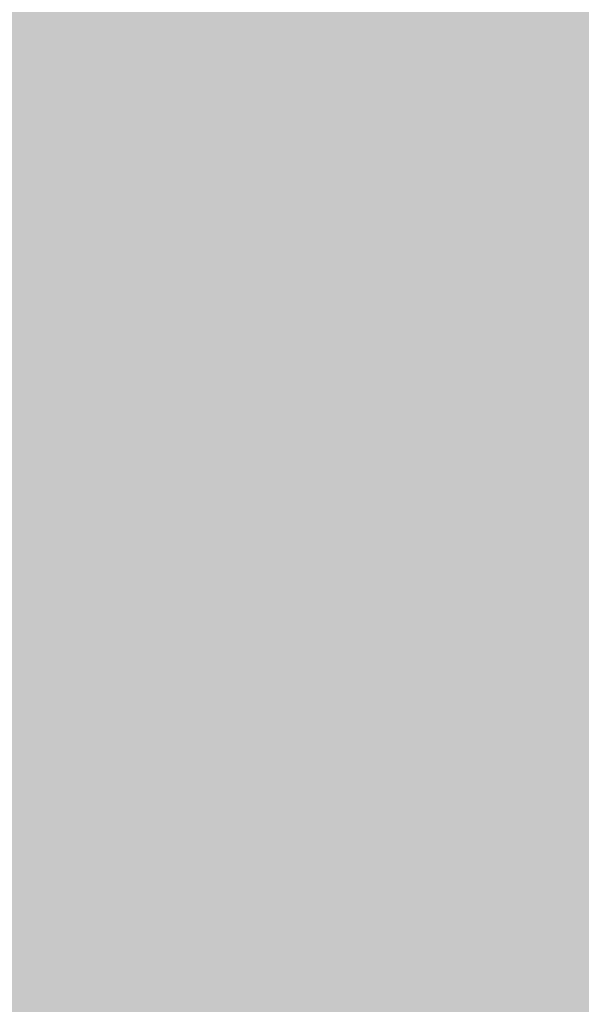
# Model space of a CAD drawing. Units: inches. Extents: x 2083 to 3317, y 1141 to 2115.
# Tile 186 of 256: x 3126.6699 to 3126.8176, y 1263.3548 to 1263.6134. Entities that reach past the tile are written whole.
import ezdxf

# ---------------------------------------------------------------- set-up
doc = ezdxf.new("R2010")
doc.units = ezdxf.units.IN
doc.layers.add('A-ANNO-DIMS', color=2, linetype='Continuous', lineweight=18)
doc.layers.add('A-WALL-PATT', color=251, linetype='Continuous', lineweight=13, true_color=0x636466)
doc.styles.get("Standard").update_dxf_attribs({"font": 'arial.ttf'})
doc.dimstyles.new('ISO-25', dxfattribs={"dimtxt": 12, "dimasz": 12, "dimexe": 1.25, "dimexo": 0.625, "dimtad": 1, "dimlunit": 3, "dimtxsty": 'Standard', "dimcen": 2.5, "dimadec": 0, "dimazin": 0, "dimtfac": 1, "dimtmove": 0, "dimatfit": 3, "dimfxl": 1, "dimarcsym": 0})

# ---------------------------------------------------------------- blocks, each defined once
blk = doc.blocks.new('*D26')
at = {"layer": 'A-ANNO-DIMS', "color": 0, "lineweight": -2, "transparency": 16777216}
for p, q in [((3088.98584, 1274.91509), (3088.98584, 1270.95196)), ((3111.24004, 1274.91509), (3111.24004, 1270.95196)), ((3076.98584, 1272.20196), (2840.26245, 1272.20196)), ((3111.24004, 1272.20196), (3088.98584, 1272.20196)), ((3123.24004, 1272.20196), (3135.24004, 1272.20196))]:
    blk.add_line(p, q, dxfattribs=at)
at = {"layer": 'A-ANNO-DIMS', "color": 0, "transparency": 16777216}
for points in [[(3076.98584, 1274.20196), (3076.98584, 1270.20196), (3088.98584, 1272.20196)], [(3123.24004, 1274.20196), (3123.24004, 1270.20196), (3111.24004, 1272.20196)]]:
    blk.add_solid(points, dxfattribs=at)
at = {"layer": 'Defpoints', "color": 0, "transparency": 16777216}
for p in [(3088.98584, 1275.54009), (3111.24004, 1275.54009), (3088.98584, 1272.20196)]:
    blk.add_point(p, dxfattribs=at)
at = {"layer": 'A-ANNO-DIMS', "color": 0, "transparency": 16777216, "insert": (2952.62415, 1279.0316), "char_height": 12, "attachment_point": 5}
blk.add_mtext('NIGHTSTAND 1\'-10 1/2" TYP.', dxfattribs=at)
blk = doc.blocks.new('*D27')
at = {"layer": 'A-ANNO-DIMS', "color": 0, "lineweight": -2, "transparency": 16777216}
for p, q in [((3114.57817, 1309.79428), (3114.57817, 1321.79428)), ((3111.86504, 1297.79428), (3115.82817, 1297.79428)), ((3114.57817, 1297.79428), (3114.57817, 1275.54009)), ((3111.86504, 1275.54009), (3115.82817, 1275.54009)), ((3114.57817, 1263.54009), (3114.57817, 1140.98859))]:
    blk.add_line(p, q, dxfattribs=at)
at = {"layer": 'A-ANNO-DIMS', "color": 0, "transparency": 16777216}
for points in [[(3112.57817, 1309.79428), (3116.57817, 1309.79428), (3114.57817, 1297.79428)], [(3112.57817, 1263.54009), (3116.57817, 1263.54009), (3114.57817, 1275.54009)]]:
    blk.add_solid(points, dxfattribs=at)
at = {"layer": 'Defpoints', "color": 0, "transparency": 16777216}
for p in [(3111.24004, 1297.79428), (3111.24004, 1275.54009), (3114.57817, 1275.54009)]:
    blk.add_point(p, dxfattribs=at)
at = {"layer": 'A-ANNO-DIMS', "color": 0, "transparency": 16777216, "insert": (3107.74853, 1196.26434), "char_height": 12, "attachment_point": 5, "rotation": 90}
blk.add_mtext('1\'-10 1/2" TYP.', dxfattribs=at)

msp = doc.modelspace()

# ---------------------------------------------------------------- hatches: boundary and pattern name
at = {"layer": 'A-WALL-PATT'}
h = msp.add_hatch(color=256, dxfattribs=at)
h.dxf.hatch_style = 1
h.paths.add_polyline_path([(3126.95978, 2020.76136), (2748.95978, 2020.76136), (2604.95978, 2020.76136), (2226.95978, 2020.76136), (2226.95978, 1702.76136), (2466.95978, 1702.76136), (2466.95978, 1582.76136), (2418.95978, 1582.76136), (2418.95978, 1477.76136), (2226.95978, 1477.76136), (2226.95978, 1263.26136), (2544.95978, 1263.26136), (2544.95978, 1411.76136), (2604.95978, 1411.76136), (2685.95978, 1411.76136), (2685.95978, 1420.76136), (2604.95978, 1420.76136), (2604.95978, 1573.76136), (2604.95978, 1702.76136), (2604.95978, 2011.76136), (2748.95978, 2011.76136), (2748.95978, 1702.76136), (2862.95978, 1702.76136), (2862.95978, 1621.76136), (2871.95978, 1621.76136), (2871.95978, 1702.76136), (2883.95978, 1702.76136), (2883.95978, 1706.93946, -0.026459), (2883.95978, 1711.76136), (2757.95978, 1711.76136), (2757.95978, 1807.76136), (2787.95978, 1807.76136), (2787.95978, 1812.26136), (2757.95978, 1812.26136), (2757.95978, 2011.76136), (2877.95978, 2011.76136), (2877.95978, 1812.26136), (2847.95978, 1812.26136), (2847.95978, 1807.76136), (2889.83574, 1807.76136), (2889.83574, 1812.26136), (2882.45978, 1812.26136), (2882.45978, 2011.76136), (3117.95978, 2011.76136), (3117.95978, 1812.26136), (2937.83574, 1812.26136), (2937.83574, 1807.76136), (2995.70978, 1807.76136), (2995.70978, 1796.11767), (3000.20978, 1796.11767), (3000.20978, 1807.76136), (3117.95978, 1807.76136), (3117.95978, 1711.76136), (3000.20978, 1711.76136), (3000.20978, 1760.11767), (2998.5727, 1760.11767, -0.020711), (2995.70978, 1760.11767), (2995.70978, 1711.76136), (2931.95978, 1711.76136), (2931.95978, 1702.76136), (3126.95978, 1702.76136)])
h.paths.add_polyline_path([(2471.45978, 2011.76136), (2471.45978, 1810.01136), (2462.71694, 1810.01136), (2462.71694, 1805.51136), (2505.95978, 1805.51136), (2505.95978, 1810.01136), (2475.95978, 1810.01136), (2475.95978, 2011.76136), (2595.95978, 2011.76136), (2595.95978, 1810.01136), (2565.95978, 1810.01136), (2565.95978, 1805.51136), (2595.95978, 1805.51136), (2595.95978, 1711.76136), (2235.95978, 1711.76136), (2235.95978, 1805.51136), (2353.70978, 1805.51136), (2353.70978, 1796.05416), (2358.20978, 1796.05416), (2358.20978, 1805.51136), (2414.71694, 1805.51136), (2414.71694, 1810.01136), (2235.95978, 1810.01136), (2235.95978, 2011.76136)], flags=16)
h.paths.add_polyline_path([(2270.20473, 1994.61001), (2270.20473, 1970.61001), (2246.20473, 1970.61001), (2246.20473, 1994.61001)], flags=0)
edge = h.paths.add_edge_path(flags=0)
edge.add_ellipse((2332.02739, 1899.79818), major_axis=(-3.04299, 3.04299), ratio=0.1682525, start_angle=-161.33217, end_angle=-156.30711, ccw=False)
edge.add_ellipse((2333.08204, 1898.74353), major_axis=(-1.05465, 1.05465), ratio=0.4535321, start_angle=-123.37102, end_angle=-94.15911)
edge = h.paths.add_edge_path(flags=0)
edge.add_ellipse((2332.02739, 1968.87629), major_axis=(3.04299, 3.04299), ratio=0.1682525, start_angle=18.66783, end_angle=23.69289)
edge.add_spline(control_points=[(2332.9256, 1970.6911), (2332.22677, 1970.3361), (2330.89371, 1969.65891), (2328.41308, 1970.93214), (2327.20393, 1967.74871), (2324.7096, 1969.95559), (2322.53282, 1967.01235), (2320.01285, 1971.29581), (2317.68031, 1968.15784), (2316.04053, 1967.10205), (2315.4269, 1966.8096)], knot_values=[0, 0, 0, 0, 2.267059, 4.324559, 6.685584, 8.878641, 11.121502, 14.300359, 17.755284, 19.732645, 19.732645, 19.732645, 19.732645], degree=3, periodic=0)
edge.add_ellipse((2332.02739, 1968.87629), major_axis=(3.04299, 3.04299), ratio=0.1682525, start_angle=18.66783, end_angle=23.69289, ccw=False)
edge.add_ellipse((2333.08204, 1969.93094), major_axis=(1.05465, 1.05465), ratio=0.4535321, start_angle=56.62898, end_angle=85.84089, ccw=False)
edge = h.paths.add_edge_path(flags=0)
edge.add_spline(control_points=[(2296.42829, 1967.98791), (2293.6278, 1965.33631), (2287.70362, 1959.72709), (2299.74386, 1949.9957), (2294.53259, 1935.66853), (2290.57323, 1920.60351), (2293.39412, 1909.97369), (2296.18541, 1904.96654)], knot_values=[0.099185, 0.099185, 0.099185, 0.099185, 0.345301, 0.619822, 0.982653, 1.386093, 1.810555, 1.810555, 1.810555, 1.810555], degree=3, periodic=0)
edge.add_spline(control_points=[(2296.18541, 1904.96654), (2297.38358, 1902.6193), (2298.00097, 1901.94931), (2298.55297, 1901.46815)], knot_values=[0.006246, 0.006246, 0.006246, 0.006246, 0.055476, 0.055476, 0.055476, 0.055476], degree=3, periodic=0)
edge.add_spline(control_points=[(2298.55297, 1901.46815), (2297.25861, 1900.92322), (2295.22529, 1900.23213), (2293.06023, 1900.61421), (2292.10142, 1900.78841), (2292.08958, 1900.79057)], knot_values=[0.312835, 0.312835, 0.312835, 0.312835, 0.40178, 0.474987, 0.475903, 0.475903, 0.475903, 0.475903], degree=3, periodic=0)
edge.add_arc((2292.79365, 1904.66411), 3.93701, 215.4209, 259.69818, ccw=False)
edge.add_spline(control_points=[(2289.58531, 1902.3823), (2289.47665, 1902.53509), (2289.36848, 1902.68804), (2289.26086, 1902.84117)], knot_values=[0.102872, 0.102872, 0.102872, 0.102872, 0.116896, 0.116896, 0.116896, 0.116896], degree=3, periodic=0)
edge.add_spline(control_points=[(2289.26086, 1902.84117), (2288.6866, 1902.55019), (2287.64005, 1902.0199), (2285.88134, 1901.87395), (2283.85297, 1901.50435), (2281.71999, 1899.71054), (2278.46699, 1899.49294), (2276.15714, 1901.8832), (2272.25895, 1899.80407), (2267.77761, 1901.84318), (2262.24388, 1900.18403), (2257.41493, 1901.78206), (2254.31837, 1900.72612), (2253.17828, 1900.33734)], knot_values=[0, 0, 0, 0, 1.907977, 3.477176, 5.261074, 7.972851, 11.680248, 13.717921, 16.939592, 22.789562, 27.502503, 33.595215, 37.145618, 37.145618, 37.145618, 37.145618], degree=3, periodic=0)
edge.add_line((2253.17828, 1900.33734), (2250.24424, 1902.84117))
edge.add_line((2250.24424, 1902.84117), (2250.24424, 1965.8333))
edge.add_line((2250.24424, 1965.8333), (2253.17828, 1968.33712))
edge.add_spline(control_points=[(2253.17828, 1968.33712), (2254.31837, 1967.94835), (2257.41493, 1966.89241), (2262.24388, 1968.49043), (2267.77761, 1966.83128), (2271.52673, 1968.53722), (2273.87591, 1967.82829), (2274.2067, 1967.72764)], knot_values=[0, 0, 0, 0, 0.09018, 0.244935, 0.364644, 0.513233, 0.537855, 0.537855, 0.537855, 0.537855], degree=3, periodic=0)
edge.add_arc((2274.35289, 1963.79335), 3.93701, 72.05113, 92.12795, ccw=False)
edge.add_arc((2281.29693, 1985.23), 18.5963, 252.051134, 288.565722)
edge.add_arc((2292.31672, 1956.02888), 12.64608, 71.026788, 113.778218, ccw=False)
edge = h.paths.add_edge_path(flags=0)
edge.add_spline(control_points=[(2274.89941, 1951.85619), (2275.06616, 1951.61659), (2275.23269, 1951.37659), (2275.39799, 1951.13585)], knot_values=[1.409916, 1.409916, 1.409916, 1.409916, 1.43159, 1.43159, 1.43159, 1.43159], degree=3, periodic=0)
edge.add_spline(control_points=[(2275.39799, 1951.13585), (2275.79211, 1950.56189), (2276.17923, 1949.98377), (2276.54555, 1949.3971)], knot_values=[1.358238, 1.358238, 1.358238, 1.358238, 1.409916, 1.409916, 1.409916, 1.409916], degree=3, periodic=0)
edge.add_line((2276.54555, 1949.3971), (2277.43729, 1947.86218))
edge.add_spline(control_points=[(2277.43729, 1947.86218), (2276.30383, 1945.67311), (2274.6397, 1942.42688), (2274.63161, 1938.0939), (2272.79912, 1930.85155), (2274.35643, 1943.89705), (2275.94768, 1947.92336), (2276.54555, 1949.3971)], knot_values=[0.005632, 0.005632, 0.005632, 0.005632, 0.186014, 0.266002, 0.357087, 0.59639, 0.739732, 0.739732, 0.739732, 0.739732], degree=3, periodic=0)
edge.add_spline(control_points=[(2276.54555, 1949.3971), (2276.17923, 1949.98377), (2275.79211, 1950.56189), (2275.39799, 1951.13585)], knot_values=[1.358238, 1.358238, 1.358238, 1.358238, 1.409916, 1.409916, 1.409916, 1.409916], degree=3, periodic=0)
edge.add_spline(control_points=[(2275.39799, 1951.13585), (2274.9425, 1950.08045), (2274.20776, 1948.02527), (2273.9346, 1944.85148), (2272.46853, 1937.62749), (2273.46622, 1945.69647), (2274.70062, 1951.05947), (2274.89941, 1951.85619)], knot_values=[0.104364, 0.104364, 0.104364, 0.104364, 0.189636, 0.269624, 0.36071, 0.600013, 0.644622, 0.644622, 0.644622, 0.644622], degree=3, periodic=0)
h.paths.add_polyline_path([(2269.16751, 1963.12757, -0.357527), (2268.17063, 1960.97637, -0.092561), (2268.17063, 1939.43632, -0.357527), (2269.16751, 1937.28512, -0.357527), (2267.01631, 1938.282, -0.164785), (2254.68558, 1938.282, -0.357527), (2252.53438, 1937.28512, -0.357527), (2253.53126, 1939.43632, -0.092561), (2253.53126, 1960.97637, -0.357527), (2252.53438, 1963.12757, -0.357527), (2254.68558, 1962.13069, -0.164785), (2267.01631, 1962.13069, -0.357527)], flags=0)
h.paths.add_polyline_path([(2248.87407, 1967.8018), (2248.87407, 1957.02771), (2249.45778, 1957.02771), (2249.45778, 1911.64676), (2248.87407, 1911.64676), (2248.87407, 1900.87267), (2246.51186, 1900.87267, 0.197327), (2244.14966, 1902.45687), (2244.14966, 1966.21759, 0.197327), (2246.51186, 1967.8018)], flags=0)
h.paths.add_polyline_path([(2269.16751, 1931.38934, -0.357527), (2268.17063, 1929.23814, -0.092561), (2268.17063, 1907.6981, -0.357527), (2269.16751, 1905.54689, -0.357527), (2267.01631, 1906.54377, -0.164785), (2254.68558, 1906.54377, -0.357527), (2252.53438, 1905.54689, -0.357527), (2253.53126, 1907.6981, -0.092561), (2253.53126, 1929.23814, -0.357527), (2252.53438, 1931.38934, -0.357527), (2254.68558, 1930.39246, -0.164785), (2267.01631, 1930.39246, -0.357527)], flags=0)
edge = h.paths.add_edge_path(flags=0)
edge.add_spline(control_points=[(2276.19686, 1906.7237), (2276.16814, 1909.02893), (2276.11405, 1913.37185), (2270.59842, 1924.92498), (2273.90517, 1919.01278), (2275.92171, 1916.26206), (2275.47457, 1912.40215), (2277.25787, 1910.38062), (2276.69604, 1908.22504), (2276.64622, 1906.81302), (2276.61782, 1906.00841)], knot_values=[0, 0, 0, 0, 8.61026, 16.221274, 18.843057, 23.804898, 27.440828, 29.356102, 31.203478, 33.650687, 33.650687, 33.650687, 33.650687], degree=3, periodic=0)
edge.add_spline(control_points=[(2276.61782, 1906.00841), (2276.62331, 1905.62414), (2276.49774, 1904.62866), (2275.44178, 1903.85473), (2274.93731, 1903.08045), (2274.85908, 1902.84117)], knot_values=[0.156488, 0.156488, 0.156488, 0.156488, 0.184398, 0.231376, 0.250598, 0.250598, 0.250598, 0.250598], degree=3, periodic=0)
edge.add_line((2274.85908, 1902.84117), (2276.50598, 1902.84117))
edge.add_spline(control_points=[(2276.50598, 1902.84117), (2276.78831, 1903.08494), (2277.66507, 1904.1252), (2278.24954, 1904.34074), (2277.65387, 1908.52739), (2278.15567, 1906.22781), (2278.10046, 1905.28595), (2278.84667, 1904.06901), (2277.85679, 1903.41495), (2277.87419, 1902.99105), (2277.90356, 1902.84117)], knot_values=[0.059574, 0.059574, 0.059574, 0.059574, 0.080753, 0.103741, 0.16972, 0.176036, 0.207137, 0.240474, 0.262341, 0.27366, 0.27366, 0.27366, 0.27366], degree=3, periodic=0)
edge.add_line((2277.90356, 1902.84117), (2280.02983, 1902.84117))
edge.add_spline(control_points=[(2280.02983, 1902.84117), (2279.88822, 1903.0884), (2279.49926, 1903.98155), (2280.15228, 1905.93935), (2278.10362, 1909.65776), (2279.76239, 1907.18529), (2280.3279, 1904.87486), (2280.48511, 1903.48959), (2281.46327, 1903.24943), (2281.75834, 1902.9365), (2281.83404, 1902.84117)], knot_values=[0.013856, 0.013856, 0.013856, 0.013856, 0.034874, 0.088867, 0.107879, 0.126738, 0.158714, 0.193757, 0.217487, 0.226722, 0.226722, 0.226722, 0.226722], degree=3, periodic=0)
edge.add_spline(control_points=[(2281.83404, 1902.84117), (2281.78753, 1902.8267), (2281.64702, 1902.78299), (2281.39553, 1902.85949), (2281.08808, 1902.98524), (2280.72068, 1903.0609), (2280.33345, 1903.02573), (2280.12477, 1902.89888), (2280.02983, 1902.84117)], knot_values=[0, 0, 0, 0, 0.14413, 0.435517, 0.749276, 1.153046, 1.548371, 1.878348, 1.878348, 1.878348, 1.878348], degree=3, periodic=0)
edge.add_line((2280.02983, 1902.84117), (2277.90356, 1902.84117))
edge.add_spline(control_points=[(2277.90356, 1902.84117), (2277.89286, 1902.79586), (2277.8654, 1902.67964), (2277.60748, 1902.68748), (2277.27405, 1902.8007), (2276.83792, 1902.61977), (2276.58381, 1902.78926), (2276.50598, 1902.84117)], knot_values=[0, 0, 0, 0, 0.127189, 0.326199, 0.628009, 1.24357, 1.515331, 1.515331, 1.515331, 1.515331], degree=3, periodic=0)
edge.add_line((2276.50598, 1902.84117), (2274.85908, 1902.84117))
edge.add_spline(control_points=[(2274.85908, 1902.84117), (2274.81444, 1902.89859), (2274.72513, 1903.01345), (2274.49348, 1903.11897), (2274.24429, 1902.96054), (2273.93712, 1903.18494), (2273.61404, 1902.98314), (2273.40832, 1902.88304), (2273.32225, 1902.84117)], knot_values=[0, 0, 0, 0, 0.21843, 0.436957, 0.687977, 0.990379, 1.398396, 1.69185, 1.69185, 1.69185, 1.69185], degree=3, periodic=0)
edge.add_spline(control_points=[(2273.32225, 1902.84117), (2273.61674, 1903.44569), (2274.274, 1904.53825), (2276.02724, 1904.5737), (2276.20696, 1906.58364), (2276.19686, 1906.7237)], knot_values=[0.012227, 0.012227, 0.012227, 0.012227, 0.059472, 0.106218, 0.134458, 0.134458, 0.134458, 0.134458], degree=3, periodic=0)
h.paths.add_polyline_path([(2270.77605, 1897.78983), (2270.77605, 1873.78983), (2246.77605, 1873.78983), (2246.77605, 1897.78983)], flags=0)
h.paths.add_polyline_path([(2353.70978, 1760.00506), (2353.70978, 1760.05416), (2358.20978, 1760.05416, -0.033729)], flags=0)
h.paths.add_polyline_path([(2321.81912, 1737.52919), (2341.99533, 1737.52919, -0.414214), (2343.20327, 1736.32124), (2343.20327, 1721.0206, -0.414214), (2341.99533, 1719.81265), (2321.81912, 1719.81265, -0.414214), (2320.61117, 1721.0206), (2320.61117, 1736.32124, -0.414214)], flags=0)
h.paths.add_polyline_path([(2324.23501, 1736.32124), (2339.57944, 1736.32124, -0.414214), (2341.99533, 1733.90535), (2341.99533, 1725.44973, -0.414214), (2339.57944, 1723.03384), (2333.68059, 1723.03384), (2333.84532, 1722.04547, -0.870646), (2335.4254, 1721.82589, -0.767327), (2333.92269, 1721.42324), (2331.29102, 1721.42324, -0.767327), (2329.78832, 1721.82589, -0.870646), (2331.3684, 1722.04547), (2331.53313, 1723.03384), (2324.23501, 1723.03384, -0.414214), (2321.81912, 1725.44973), (2321.81912, 1733.90535, -0.414214)], flags=0)
h.paths.add_polyline_path([(2570.48379, 1928.61544), (2589.68379, 1928.61544), (2590.16883, 1928.61544), (2590.16883, 1904.9934), (2570.48379, 1904.9934)], flags=0)
h.paths.add_polyline_path([(2574.44732, 1927.26382, -1), (2572.82884, 1927.26382, -1)], flags=0)
h.paths.add_polyline_path([(2573.08987, 1926.94088), (2573.92503, 1927.77604), (2574.14774, 1927.55333), (2573.31258, 1926.71817)], flags=0)
h.paths.add_polyline_path([(2578.77906, 1919.72962, -1), (2571.59166, 1919.72962, -1)], flags=0)
h.paths.add_polyline_path([(2578.38536, 1919.72962, -1), (2571.98536, 1919.72962, -1)], flags=0)
h.paths.add_polyline_path([(2331.59576, 1729.47622, -1), (2333.61795, 1729.47622, -1)], flags=0)
h.paths.add_polyline_path([(2578.03423, 1927.26382, -1), (2576.41574, 1927.26382, -1)], flags=0)
h.paths.add_polyline_path([(2576.68885, 1927.53109), (2576.91156, 1927.7538), (2577.74673, 1926.91863), (2577.52402, 1926.69592)], flags=0)
h.paths.add_polyline_path([(2578.13906, 1909.85954, -1), (2572.23166, 1909.85954, -1)], flags=0)
h.paths.add_polyline_path([(2577.74536, 1909.85954, -1), (2572.62536, 1909.85954, -1)], flags=0)
h.paths.add_polyline_path([(2583.79772, 1927.26382, -1), (2582.17923, 1927.26382, -1)], flags=0)
h.paths.add_polyline_path([(2582.71865, 1927.7538), (2583.55381, 1926.91863), (2583.3311, 1926.69592), (2582.49594, 1927.53109)], flags=0)
h.paths.add_polyline_path([(2582.49594, 1927.53109), (2582.71865, 1927.7538), (2583.55381, 1926.91863), (2583.3311, 1926.69592)], flags=0)
h.paths.add_polyline_path([(2587.73906, 1920.52962, -1), (2581.83166, 1920.52962, -1)], flags=0)
h.paths.add_polyline_path([(2587.34536, 1920.52962, -1), (2582.22536, 1920.52962, -1)], flags=0)
h.paths.add_polyline_path([(2587.38462, 1927.26382, -1), (2585.76613, 1927.26382, -1)], flags=0)
h.paths.add_polyline_path([(2586.08199, 1926.98025), (2586.91716, 1927.81541), (2587.13987, 1927.5927), (2586.3047, 1926.75754)], flags=0)
h.paths.add_polyline_path([(2588.37906, 1910.65954, -1), (2581.19166, 1910.65954, -1)], flags=0)
h.paths.add_polyline_path([(2587.98536, 1910.65954, -1), (2581.58536, 1910.65954, -1)], flags=0)
h.paths.add_polyline_path([(2417.16773, 1729.4779), (2437.34394, 1729.4779, -0.414214), (2438.55188, 1728.26995), (2438.55188, 1712.96931, -0.414214), (2437.34394, 1711.76136), (2417.16773, 1711.76136, -0.414214), (2415.95978, 1712.96931), (2415.95978, 1728.26995, -0.414214)], flags=0)
h.paths.add_polyline_path([(2419.58362, 1728.26995), (2434.92805, 1728.26995, -0.414214), (2437.34394, 1725.85406), (2437.34394, 1717.39844, -0.414214), (2434.92805, 1714.98255), (2429.0292, 1714.98255), (2429.19393, 1713.99418, -0.870646), (2430.77401, 1713.7746, -0.767327), (2429.2713, 1713.37195), (2426.63963, 1713.37195, -0.767327), (2425.13693, 1713.7746, -0.870646), (2426.71701, 1713.99418), (2426.88174, 1714.98255), (2419.58362, 1714.98255, -0.414214), (2417.16773, 1717.39844), (2417.16773, 1725.85406, -0.414214)], flags=0)
h.paths.add_polyline_path([(2419.58362, 1728.26995), (2434.92805, 1728.26995, -0.414214), (2437.34394, 1725.85406), (2437.34394, 1717.39844, -0.414214), (2434.92805, 1714.98255), (2429.0292, 1714.98255), (2428.35812, 1719.00903), (2427.55282, 1719.00903), (2426.88174, 1714.98255), (2419.58362, 1714.98255, -0.414214), (2417.16773, 1717.39844), (2417.16773, 1725.85406, -0.414214)], flags=0)
h.paths.add_polyline_path([(2426.94437, 1721.42492, -1), (2428.96656, 1721.42492, -1)], flags=0)
h.paths.add_polyline_path([(2475.95978, 1702.76136), (2595.95978, 1702.76136), (2595.95978, 1582.76136), (2475.95978, 1582.76136)], flags=16)
h.paths.add_polyline_path([(2427.95978, 1573.76136), (2595.95978, 1573.76136), (2595.95978, 1468.76136), (2595.95978, 1420.76136), (2384.45978, 1420.76136), (2384.45978, 1468.76136), (2427.95978, 1468.76136)], flags=16)
h.paths.add_polyline_path([(2379.95978, 1468.76136), (2379.95978, 1420.76136), (2235.95978, 1420.76136), (2235.95978, 1468.76136)], flags=16)
h.paths.add_polyline_path([(2317.816, 1466.69577), (2337.9922, 1466.69577, -0.414214), (2339.20015, 1465.48782), (2339.20015, 1450.18718, -0.414214), (2337.9922, 1448.97923), (2317.816, 1448.97923, -0.414214), (2316.60805, 1450.18718), (2316.60805, 1465.48782, -0.414214)], flags=0)
h.paths.add_polyline_path([(2320.23189, 1465.48782), (2335.57631, 1465.48782, -0.414214), (2337.9922, 1463.07193), (2337.9922, 1454.61631, -0.414214), (2335.57631, 1452.20042), (2329.67747, 1452.20042), (2329.84219, 1451.21205, -0.870646), (2331.42228, 1450.99247, -0.767327), (2329.91957, 1450.58983), (2327.2879, 1450.58983, -0.767327), (2325.7852, 1450.99247, -0.870646), (2327.36528, 1451.21205), (2327.53001, 1452.20042), (2320.23189, 1452.20042, -0.414214), (2317.816, 1454.61631), (2317.816, 1463.07193, -0.414214)], flags=0)
h.paths.add_polyline_path([(2320.23189, 1465.48782), (2335.57631, 1465.48782, -0.414214), (2337.9922, 1463.07193), (2337.9922, 1454.61631, -0.414214), (2335.57631, 1452.20042), (2329.67747, 1452.20042), (2329.00638, 1456.22691), (2328.20109, 1456.22691), (2327.53001, 1452.20042), (2320.23189, 1452.20042, -0.414214), (2317.816, 1454.61631), (2317.816, 1463.07193, -0.414214)], flags=0)
h.paths.add_polyline_path([(2327.59264, 1458.6428, -1), (2329.61483, 1458.6428, -1)], flags=0)
h.paths.add_polyline_path([(2244.41174, 1433.34045), (2241.92094, 1433.34045, -0.414214), (2240.01786, 1435.24354), (2240.01786, 1440.95281, -0.414211), (2241.92093, 1442.8559), (2244.41174, 1442.8559, -1.976472)], flags=0)
h.paths.add_polyline_path([(2245.35689, 1434.39754, -0.414214), (2245.35689, 1441.79881, -2.144098)], flags=0)
h.paths.add_polyline_path([(2535.95978, 1416.26136), (2535.95978, 1272.26136), (2235.95978, 1272.26136), (2235.95978, 1416.26136)], flags=16)
h.paths.add_polyline_path([(2260.11956, 1384.29284), (2260.11956, 1362.03865), (2237.86537, 1362.03865), (2237.86537, 1384.29284)], flags=0)
edge = h.paths.add_edge_path(flags=0)
edge.add_line((2318.25185, 1362.0933), (2318.1458, 1362.00097))
edge.add_ellipse((2317.44512, 1360.43104), major_axis=(2.82164, 2.82164), ratio=0.1682525, start_angle=18.66783, end_angle=20.94813, ccw=False)
edge.add_ellipse((2318.42305, 1361.40897), major_axis=(0.97793, 0.97793), ratio=0.4535321, start_angle=56.62898, end_angle=70.2262, ccw=False)
edge = h.paths.add_edge_path(flags=0)
edge.add_line((2319.10737, 1295.57108), (2319.01504, 1295.67713))
edge.add_ellipse((2317.44512, 1296.37781), major_axis=(-2.82164, 2.82164), ratio=0.1682525, start_angle=-161.33217, end_angle=-159.05187, ccw=False)
edge.add_ellipse((2318.42305, 1295.39988), major_axis=(-0.97793, 0.97793), ratio=0.4535321, start_angle=-123.37102, end_angle=-109.7738)
edge = h.paths.add_edge_path(flags=0)
edge.add_spline(control_points=[(2284.21035, 1301.17022), (2284.58069, 1300.44472), (2284.89119, 1299.89202), (2285.15955, 1299.46102)], knot_values=[0.039066, 0.039066, 0.039066, 0.039066, 0.055476, 0.055476, 0.055476, 0.055476], degree=3, periodic=0)
edge.add_line((2285.15955, 1299.46102), (2284.21035, 1301.17022))
edge = h.paths.add_edge_path(flags=0)
edge.add_line((2280.41246, 1297.29801), (2283.36999, 1297.03612))
edge.add_line((2283.36999, 1297.03612), (2286.40569, 1297.92631))
edge.add_spline(control_points=[(2286.40569, 1297.92631), (2285.30549, 1297.46312), (2284.34478, 1297.12915), (2283.36999, 1297.03612)], knot_values=[0.394369, 0.394369, 0.394369, 0.394369, 0.475903, 0.475903, 0.475903, 0.475903], degree=3, periodic=0)
edge.add_spline(control_points=[(2283.36999, 1297.03612), (2283.28139, 1297.02767), (2282.31629, 1296.95734), (2281.3125, 1297.13448), (2280.42344, 1297.29602), (2280.41246, 1297.29801)], knot_values=[0.312835, 0.312835, 0.312835, 0.312835, 0.320246, 0.393453, 0.394369, 0.394369, 0.394369, 0.394369], degree=3, periodic=0)
edge = h.paths.add_edge_path(flags=0)
edge.add_line((2284.43556, 1359.60729), (2280.44629, 1355.32805))
edge.add_line((2280.44629, 1355.32805), (2279.57999, 1351.01775))
edge.add_line((2279.57999, 1351.01775), (2282.41297, 1346.58043))
edge.add_spline(control_points=[(2282.41297, 1346.58043), (2283.15333, 1345.58924), (2284.2529, 1344.0289), (2284.80104, 1342.38717), (2284.93516, 1341.80554)], knot_values=[1.240098, 1.240098, 1.240098, 1.240098, 1.332892, 1.382712, 1.382712, 1.382712, 1.382712], degree=3, periodic=0)
edge.add_spline(control_points=[(2284.93516, 1341.80554), (2285.31911, 1340.1406), (2285.23303, 1338.4092), (2284.90994, 1336.65412)], knot_values=[1.097484, 1.097484, 1.097484, 1.097484, 1.240098, 1.240098, 1.240098, 1.240098], degree=3, periodic=0)
edge.add_spline(control_points=[(2284.90994, 1336.65412), (2284.58685, 1334.89904), (2284.02675, 1333.12027), (2283.46264, 1331.36058)], knot_values=[0.95487, 0.95487, 0.95487, 0.95487, 1.097484, 1.097484, 1.097484, 1.097484], degree=3, periodic=0)
edge.add_line((2283.46264, 1331.36058), (2281.89038, 1326.15336))
edge.add_line((2281.89038, 1326.15336), (2280.75626, 1321.05609))
edge.add_line((2280.75626, 1321.05609), (2280.2992, 1316.00198))
edge.add_line((2280.2992, 1316.00198), (2280.71593, 1310.95007))
edge.add_line((2280.71593, 1310.95007), (2282.02809, 1305.97214))
edge.add_line((2282.02809, 1305.97214), (2284.21035, 1301.17022))
edge.add_spline(control_points=[(2284.21035, 1301.17022), (2283.34073, 1302.73019), (2282.6119, 1304.33649), (2282.02809, 1305.97214)], knot_values=[0.099185, 0.099185, 0.099185, 0.099185, 0.241799, 0.241799, 0.241799, 0.241799], degree=3, periodic=0)
edge.add_spline(control_points=[(2282.02809, 1305.97214), (2281.44428, 1307.60778), (2281.00549, 1309.27276), (2280.71593, 1310.95007)], knot_values=[0.241799, 0.241799, 0.241799, 0.241799, 0.384413, 0.384413, 0.384413, 0.384413], degree=3, periodic=0)
edge.add_spline(control_points=[(2280.71593, 1310.95007), (2280.43324, 1312.58761), (2280.28939, 1314.27696), (2280.29889, 1315.96203), (2280.2992, 1316.00198)], knot_values=[0.384413, 0.384413, 0.384413, 0.384413, 0.523647, 0.527028, 0.527028, 0.527028, 0.527028], degree=3, periodic=0)
edge.add_spline(control_points=[(2280.2992, 1316.00198), (2280.31233, 1317.68696), (2280.47787, 1319.36793), (2280.75626, 1321.05609)], knot_values=[0.527028, 0.527028, 0.527028, 0.527028, 0.669642, 0.669642, 0.669642, 0.669642], degree=3, periodic=0)
edge.add_spline(control_points=[(2280.75626, 1321.05609), (2281.03465, 1322.74425), (2281.42588, 1324.43961), (2281.89038, 1326.15336)], knot_values=[0.669642, 0.669642, 0.669642, 0.669642, 0.812256, 0.812256, 0.812256, 0.812256], degree=3, periodic=0)
edge.add_spline(control_points=[(2281.89038, 1326.15336), (2282.26438, 1327.53325), (2282.78787, 1329.26181), (2283.35275, 1331.01778), (2283.46264, 1331.36058)], knot_values=[0.812256, 0.812256, 0.812256, 0.812256, 0.927087, 0.95487, 0.95487, 0.95487, 0.95487], degree=3, periodic=0)
edge.add_line((2283.46264, 1331.36058), (2284.90994, 1336.65412))
edge.add_line((2284.90994, 1336.65412), (2284.93516, 1341.80554))
edge.add_line((2284.93516, 1341.80554), (2282.41297, 1346.58043))
edge.add_spline(control_points=[(2282.41297, 1346.58043), (2281.27513, 1348.10379), (2280.07845, 1349.57032), (2279.57999, 1351.01775)], knot_values=[1.382712, 1.382712, 1.382712, 1.382712, 1.525326, 1.525326, 1.525326, 1.525326], degree=3, periodic=0)
edge.add_spline(control_points=[(2279.57999, 1351.01775), (2279.44328, 1351.41472), (2279.13631, 1352.85692), (2279.73519, 1354.29039), (2280.44629, 1355.32805)], knot_values=[1.525326, 1.525326, 1.525326, 1.525326, 1.564439, 1.667941, 1.667941, 1.667941, 1.667941], degree=3, periodic=0)
edge.add_spline(control_points=[(2280.44629, 1355.32805), (2281.42611, 1356.75784), (2282.93084, 1358.18256), (2284.43556, 1359.60729)], knot_values=[1.667941, 1.667941, 1.667941, 1.667941, 1.810555, 1.810555, 1.810555, 1.810555], degree=3, periodic=0)
edge.add_arc((2280.62307, 1348.51818), 11.72618, 71.026788, 113.778218)
edge.add_arc((2270.40489, 1375.59516), 17.24357, 252.051134, 288.565722, ccw=False)
edge.add_arc((2263.96597, 1355.71785), 3.65062, 72.05113, 92.12795)
edge.add_arc((2263.96597, 1355.71785), 3.65062, 92.12795, 177.98513)
edge.add_spline(control_points=[(2260.3176, 1355.8462), (2260.26042, 1354.22067), (2260.55128, 1350.18655), (2262.99934, 1346.76625), (2264.47274, 1344.64902)], knot_values=[1.43159, 1.43159, 1.43159, 1.43159, 1.564144, 1.770695, 1.770695, 1.770695, 1.770695], degree=3, periodic=0)
edge.add_line((2264.47274, 1344.64902), (2264.93559, 1343.98253))
edge.add_spline(control_points=[(2263.80104, 1340.24811), (2263.84324, 1340.51409), (2264.06724, 1341.75647), (2264.51269, 1343.00245), (2264.93505, 1343.98108)], knot_values=[0.53657, 0.53657, 0.53657, 0.53657, 0.559349, 0.644622, 0.644622, 0.644622, 0.644622], degree=3, periodic=0)
edge.add_spline(control_points=[(2264.93505, 1343.98108), (2265.11777, 1343.71497), (2265.29888, 1343.44791), (2265.47676, 1343.17936)], knot_values=[1.384077, 1.384077, 1.384077, 1.384077, 1.409916, 1.409916, 1.409916, 1.409916], degree=3, periodic=0)
edge.add_spline(control_points=[(2265.47676, 1343.17936), (2265.65464, 1342.91082), (2265.8293, 1342.64081), (2265.99913, 1342.36881)], knot_values=[1.358238, 1.358238, 1.358238, 1.358238, 1.384077, 1.384077, 1.384077, 1.384077], degree=3, periodic=0)
edge.add_line((2265.99913, 1342.36881), (2266.82601, 1340.94555))
edge.add_spline(control_points=[(2266.82601, 1340.94555), (2268.8944, 1337.08969), (2271.39817, 1325.843), (2270.51616, 1310.56856), (2275.91938, 1301.86061), (2277.78951, 1299.19945)], knot_values=[0.116896, 0.116896, 0.116896, 0.116896, 0.472987, 1.050969, 1.313793, 1.313793, 1.313793, 1.313793], degree=3, periodic=0)
edge.add_spline(control_points=[(2277.78951, 1299.19945), (2277.83941, 1299.12845), (2277.88943, 1299.0575), (2277.93957, 1298.98658)], knot_values=[0.109884, 0.109884, 0.109884, 0.109884, 0.116896, 0.116896, 0.116896, 0.116896], degree=3, periodic=0)
edge.add_line((2277.93957, 1298.98658), (2277.78885, 1299.19911))
edge.add_spline(control_points=[(2277.78885, 1299.19911), (2277.25658, 1298.92941), (2276.28635, 1298.4379), (2275.03935, 1298.33442), (2274.38333, 1298.2389), (2274.21525, 1298.20934)], knot_values=[33.12187, 33.12187, 33.12187, 33.12187, 35.029056, 36.598255, 37.144827, 37.144827, 37.144827, 37.144827], degree=3, periodic=0)
edge.add_line((2274.21525, 1298.20934), (2273.07315, 1297.89296))
edge.add_spline(control_points=[(2273.07315, 1297.89296), (2272.32294, 1297.57978), (2271.03915, 1296.51051), (2269.24839, 1296.22606), (2268.4231, 1296.37465)], knot_values=[26.532584, 26.532584, 26.532584, 26.532584, 29.198919, 31.839101, 31.839101, 31.839101, 31.839101], degree=3, periodic=0)
edge.add_line((2268.4231, 1296.37465), (2263.8785, 1297.45753))
edge.add_spline(control_points=[(2263.8785, 1297.45753), (2263.55608, 1297.35943), (2261.86031, 1296.83869), (2260.23878, 1297.28241), (2258.93345, 1297.51646)], knot_values=[15.919551, 15.919551, 15.919551, 15.919551, 16.939592, 21.226067, 21.226067, 21.226067, 21.226067], degree=3, periodic=0)
edge.add_line((2258.93345, 1297.51646), (2254.05523, 1297.32901))
edge.add_spline(control_points=[(2254.05523, 1297.32901), (2253.75553, 1297.29582), (2252.11368, 1297.16517), (2250.46187, 1297.54422), (2249.12969, 1297.66788)], knot_values=[5.306517, 5.306517, 5.306517, 5.306517, 6.276435, 10.613034, 10.613034, 10.613034, 10.613034], degree=3, periodic=0)
edge.add_line((2249.12969, 1297.66788), (2244.33165, 1296.87776))
edge.add_line((2244.33165, 1296.87776), (2241.61103, 1299.19945))
edge.add_line((2241.61103, 1299.19945), (2241.61103, 1357.6094))
edge.add_line((2241.61103, 1357.6094), (2244.33165, 1359.9311))
edge.add_line((2244.33165, 1359.9311), (2252.72882, 1359.54269))
edge.add_spline(control_points=[(2252.72882, 1359.54269), (2252.87094, 1359.54644), (2253.30574, 1359.54817), (2253.73984, 1359.51427), (2254.03174, 1359.48243)], knot_values=[0.233291, 0.233291, 0.233291, 0.233291, 0.244935, 0.268927, 0.268927, 0.268927, 0.268927], degree=3, periodic=0)
edge.add_line((2254.03174, 1359.48243), (2259.58719, 1359.41639))
edge.add_spline(control_points=[(2259.58719, 1359.41639), (2260.67707, 1359.6285), (2262.0732, 1359.897), (2263.52369, 1359.45928), (2263.83042, 1359.36595)], knot_values=[0.422516, 0.422516, 0.422516, 0.422516, 0.513233, 0.537855, 0.537855, 0.537855, 0.537855], degree=3, periodic=0)
edge.add_arc((2263.96597, 1355.71785), 3.65062, 72.05113, 92.12795, ccw=False)
edge.add_arc((2270.40489, 1375.59516), 17.24357, 252.051134, 288.565722)
edge.add_arc((2280.62307, 1348.51818), 11.72618, 71.026788, 113.778218, ccw=False)
h.paths.add_polyline_path([(2240.34053, 1359.43471), (2240.34053, 1349.44435), (2240.88178, 1349.44435), (2240.88178, 1307.3645), (2240.34053, 1307.3645), (2240.34053, 1297.37414), (2238.15016, 1297.37414, 0.197327), (2235.95978, 1298.84311), (2235.95978, 1357.96575, 0.197327), (2238.15016, 1359.43471)], flags=0)
h.paths.add_polyline_path([(2259.15779, 1355.1005, -0.357527), (2258.23342, 1353.10578, -0.092561), (2258.23342, 1333.1326, -0.357527), (2259.15779, 1331.13788, -0.357527), (2257.16307, 1332.06225, -0.164785), (2245.7293, 1332.06225, -0.357527), (2243.73458, 1331.13788, -0.357527), (2244.65895, 1333.1326, -0.092561), (2244.65895, 1353.10578, -0.357527), (2243.73458, 1355.1005, -0.357527), (2245.7293, 1354.17613, -0.164785), (2257.16307, 1354.17613, -0.357527)], flags=0)
edge = h.paths.add_edge_path(flags=0)
edge.add_line((2265.99913, 1342.36881), (2266.82601, 1340.94555))
edge.add_line((2266.82601, 1340.94555), (2265.30756, 1337.81407))
edge.add_line((2265.30756, 1337.81407), (2264.35823, 1334.65294))
edge.add_line((2264.35823, 1334.65294), (2264.26201, 1333.7997))
edge.add_spline(control_points=[(2264.26201, 1333.7997), (2264.20836, 1333.18705), (2264.16206, 1332.36553), (2264.00714, 1331.41393), (2263.96905, 1331.20183)], knot_values=[0.464444, 0.464444, 0.464444, 0.464444, 0.516691, 0.531608, 0.531608, 0.531608, 0.531608], degree=3, periodic=0)
edge.add_spline(control_points=[(2263.96905, 1331.20183), (2263.77453, 1330.11887), (2263.42437, 1328.79084), (2263.25742, 1328.53065), (2263.23403, 1328.51461)], knot_values=[0.372682, 0.372682, 0.372682, 0.372682, 0.44885, 0.464444, 0.464444, 0.464444, 0.464444], degree=3, periodic=0)
edge.add_spline(control_points=[(2263.23403, 1328.51461), (2263.09638, 1328.42023), (2263.13117, 1329.30148), (2263.27495, 1330.61575)], knot_values=[0.280919, 0.280919, 0.280919, 0.280919, 0.372682, 0.372682, 0.372682, 0.372682], degree=3, periodic=0)
edge.add_spline(control_points=[(2263.27495, 1330.61575), (2263.41874, 1331.93002), (2263.67152, 1333.67732), (2263.96985, 1335.31503)], knot_values=[0.189157, 0.189157, 0.189157, 0.189157, 0.280919, 0.280919, 0.280919, 0.280919], degree=3, periodic=0)
edge.add_spline(control_points=[(2263.96985, 1335.31503), (2264.1005, 1336.03219), (2264.41878, 1337.62191), (2264.75485, 1338.86443), (2264.94742, 1339.49112)], knot_values=[0.097394, 0.097394, 0.097394, 0.097394, 0.137578, 0.189157, 0.189157, 0.189157, 0.189157], degree=3, periodic=0)
edge.add_spline(control_points=[(2264.94742, 1339.49112), (2265.29002, 1340.60605), (2265.64424, 1341.494), (2265.99913, 1342.36881)], knot_values=[0.005632, 0.005632, 0.005632, 0.005632, 0.097394, 0.097394, 0.097394, 0.097394], degree=3, periodic=0)
h.paths.add_polyline_path([(2259.15779, 1325.67097, -0.357527), (2258.23342, 1323.67625, -0.092561), (2258.23342, 1303.70307, -0.357527), (2259.15779, 1301.70835, -0.357527), (2257.16307, 1302.63272, -0.164785), (2245.7293, 1302.63272, -0.357527), (2243.73458, 1301.70835, -0.357527), (2244.65895, 1303.70307, -0.092561), (2244.65895, 1323.67625, -0.357527), (2243.73458, 1325.67097, -0.357527), (2245.7293, 1324.74661, -0.164785), (2257.16307, 1324.74661, -0.357527)], flags=0)
edge = h.paths.add_edge_path(flags=0)
edge.add_spline(control_points=[(2261.70894, 1317.31142), (2261.67948, 1317.41758), (2261.76186, 1317.38853), (2262.49074, 1316.08987), (2262.96218, 1315.3009)], knot_values=[14.955861, 14.955861, 14.955861, 14.955861, 16.221274, 18.694826, 18.694826, 18.694826, 18.694826], degree=3, periodic=0)
edge.add_spline(control_points=[(2262.96218, 1315.3009), (2262.99044, 1315.25362), (2263.7021, 1314.06738), (2264.34898, 1313.12715), (2264.73005, 1312.16415)], knot_values=[18.694826, 18.694826, 18.694826, 18.694826, 18.843057, 22.433791, 22.433791, 22.433791, 22.433791], degree=3, periodic=0)
edge.add_spline(control_points=[(2264.73005, 1312.16415), (2264.87556, 1311.79644), (2265.17687, 1310.76981), (2265.14307, 1309.55926), (2265.24774, 1308.82419)], knot_values=[22.433791, 22.433791, 22.433791, 22.433791, 23.804898, 26.172756, 26.172756, 26.172756, 26.172756], degree=3, periodic=0)
edge.add_line((2265.24774, 1308.82419), (2265.85077, 1307.17189))
edge.add_spline(control_points=[(2265.85077, 1307.17189), (2266.06502, 1306.82168), (2266.38439, 1306.33225), (2266.4244, 1305.78055), (2266.42037, 1305.61122)], knot_values=[28.062562, 28.062562, 28.062562, 28.062562, 29.356102, 29.911721, 29.911721, 29.911721, 29.911721], degree=3, periodic=0)
edge.add_spline(control_points=[(2266.42037, 1305.61122), (2266.41612, 1305.43259), (2266.394, 1305.25), (2266.36478, 1305.06586)], knot_values=[29.911721, 29.911721, 29.911721, 29.911721, 30.497837, 30.497837, 30.497837, 30.497837], degree=3, periodic=0)
edge.add_line((2266.36478, 1305.06586), (2266.06615, 1302.1363))
edge.add_spline(control_points=[(2266.06615, 1302.1363), (2266.07124, 1301.77998), (2265.99808, 1301.19998), (2265.66327, 1300.75896), (2265.50891, 1300.58588)], knot_values=[0.156488, 0.156488, 0.156488, 0.156488, 0.184398, 0.203543, 0.203543, 0.203543, 0.203543], degree=3, periodic=0)
edge.add_line((2265.50891, 1300.58588), (2264.43534, 1299.19945))
edge.add_line((2264.43534, 1299.19945), (2265.96244, 1299.19945))
edge.add_line((2265.96244, 1299.19945), (2267.33599, 1301.17528))
edge.add_line((2267.33599, 1301.17528), (2267.31167, 1301.98624))
edge.add_spline(control_points=[(2267.31167, 1301.98624), (2267.26111, 1302.8624), (2267.16021, 1303.73713), (2267.27149, 1303.3259)], knot_values=[0.126229, 0.126229, 0.126229, 0.126229, 0.166617, 0.166617, 0.166617, 0.166617], degree=3, periodic=0)
edge.add_spline(control_points=[(2267.27149, 1303.3259), (2267.28003, 1303.2943), (2267.30979, 1303.17537), (2267.37345, 1302.88361), (2267.40612, 1302.68283), (2267.41793, 1302.60103)], knot_values=[0.166617, 0.166617, 0.166617, 0.166617, 0.16972, 0.176036, 0.180765, 0.180765, 0.180765, 0.180765], degree=3, periodic=0)
edge.add_spline(control_points=[(2267.74389, 1300.9875), (2267.68758, 1301.15094), (2267.48052, 1301.65666), (2267.48375, 1302.14479), (2267.41793, 1302.60103)], knot_values=[0.180765, 0.180765, 0.180765, 0.180765, 0.193767, 0.220139, 0.220139, 0.220139, 0.220139], degree=3, periodic=0)
edge.add_line((2267.41793, 1302.60103), (2267.74389, 1300.9875))
edge.add_spline(control_points=[(2267.74389, 1300.9875), (2267.83196, 1300.73188), (2267.93202, 1300.3099), (2267.55484, 1299.97452), (2267.42937, 1299.82921)], knot_values=[0.220139, 0.220139, 0.220139, 0.220139, 0.240474, 0.25489, 0.25489, 0.25489, 0.25489], degree=3, periodic=0)
edge.add_line((2267.42937, 1299.82921), (2267.25836, 1299.19945))
edge.add_line((2267.25836, 1299.19945), (2269.22996, 1299.19945))
edge.add_spline(control_points=[(2269.22996, 1299.19945), (2269.09865, 1299.42869), (2268.84277, 1300.01625), (2269.01157, 1300.91592), (2268.9468, 1301.66074)], knot_values=[0.013856, 0.013856, 0.013856, 0.013856, 0.034874, 0.067073, 0.067073, 0.067073, 0.067073], degree=3, periodic=0)
edge.add_line((2268.9468, 1301.66074), (2268.43158, 1303.60311))
edge.add_spline(control_points=[(2268.43158, 1303.60311), (2268.1756, 1304.19237), (2267.59621, 1305.2513), (2268.0407, 1304.62321), (2268.25139, 1304.28242)], knot_values=[0.090155, 0.090155, 0.090155, 0.090155, 0.107879, 0.120289, 0.120289, 0.120289, 0.120289], degree=3, periodic=0)
edge.add_spline(control_points=[(2268.25139, 1304.28242), (2268.36088, 1304.10533), (2269.05775, 1302.91798), (2269.38269, 1301.59042), (2269.52141, 1300.77593), (2269.57522, 1300.55578)], knot_values=[0.120289, 0.120289, 0.120289, 0.120289, 0.126738, 0.158714, 0.173506, 0.173506, 0.173506, 0.173506], degree=3, periodic=0)
edge.add_line((2269.57522, 1300.55578), (2270.6858, 1299.42126))
edge.add_spline(control_points=[(2270.6858, 1299.42126), (2270.76722, 1299.35725), (2270.83785, 1299.2814), (2270.90292, 1299.19945)], knot_values=[0.21816, 0.21816, 0.21816, 0.21816, 0.226722, 0.226722, 0.226722, 0.226722], degree=3, periodic=0)
edge.add_line((2270.9372, 1299.19291), (2270.90292, 1299.19945))
edge.add_spline(control_points=[(2270.90292, 1299.19945), (2270.85981, 1299.18603), (2270.72951, 1299.1455), (2270.49631, 1299.21644), (2270.27166, 1299.30832), (2270.12102, 1299.34796), (2270.06334, 1299.35956)], knot_values=[0.939174, 0.939174, 0.939174, 0.939174, 1.083304, 1.374691, 1.68845, 1.878348, 1.878348, 1.878348, 1.878348], degree=3, periodic=0)
edge.add_line((2270.06334, 1299.35956), (2269.22996, 1299.19945))
edge.add_line((2269.22996, 1299.19945), (2267.25836, 1299.19945))
edge.add_spline(control_points=[(2267.25836, 1299.19945), (2267.24843, 1299.15743), (2267.22297, 1299.04967), (2266.98382, 1299.05694), (2266.80921, 1299.11623), (2266.6769, 1299.10909), (2266.63653, 1299.10481)], knot_values=[0.757665, 0.757665, 0.757665, 0.757665, 0.884854, 1.083864, 1.385675, 1.515331, 1.515331, 1.515331, 1.515331], degree=3, periodic=0)
edge.add_spline(control_points=[(2266.63653, 1299.10481), (2266.48522, 1299.08879), (2266.23581, 1299.01712), (2266.03461, 1299.15132), (2265.96244, 1299.19945)], knot_values=[0, 0, 0, 0, 0.485905, 0.757665, 0.757665, 0.757665, 0.757665], degree=3, periodic=0)
edge.add_line((2265.96244, 1299.19945), (2264.43534, 1299.19945))
edge.add_line((2264.43534, 1299.19945), (2263.85844, 1299.36712))
edge.add_spline(control_points=[(2263.85844, 1299.36712), (2263.81894, 1299.37091), (2263.77953, 1299.38572), (2263.74013, 1299.4015)], knot_values=[0.845925, 0.845925, 0.845925, 0.845925, 0.978627, 0.978627, 0.978627, 0.978627], degree=3, periodic=0)
edge.add_line((2263.72179, 1299.39643), (2263.01031, 1299.19945))
edge.add_spline(control_points=[(2263.01031, 1299.19945), (2263.24579, 1299.68286), (2263.50603, 1300.12811), (2263.87349, 1300.40803)], knot_values=[0.012227, 0.012227, 0.012227, 0.012227, 0.052971, 0.052971, 0.052971, 0.052971], degree=3, periodic=0)
edge.add_spline(control_points=[(2263.87349, 1300.40803), (2263.93213, 1300.4527), (2264.08424, 1300.55298), (2264.25519, 1300.62422), (2264.35969, 1300.66475)], knot_values=[0.052971, 0.052971, 0.052971, 0.052971, 0.059472, 0.069086, 0.069086, 0.069086, 0.069086], degree=3, periodic=0)
edge.add_line((2264.35969, 1300.66475), (2265.1419, 1301.07777))
edge.add_line((2265.1419, 1301.07777), (2265.67581, 1302.79956))
edge.add_line((2265.67581, 1302.79956), (2265.5407, 1305.70407))
edge.add_line((2265.5407, 1305.70407), (2264.80307, 1309.32772))
edge.add_line((2264.80307, 1309.32772), (2263.04053, 1314.09179))
edge.add_spline(control_points=[(2263.04053, 1314.09179), (2262.38357, 1315.67144), (2261.79597, 1316.99775), (2261.70894, 1317.31142)], knot_values=[11.216896, 11.216896, 11.216896, 11.216896, 14.955861, 14.955861, 14.955861, 14.955861], degree=3, periodic=0)
h.paths.add_polyline_path([(2871.95978, 1416.26136), (2895.91005, 1416.26136), (2895.91005, 1420.76136), (2871.95978, 1420.76136), (2871.95978, 1501.76136), (2862.95978, 1501.76136), (2862.95978, 1420.76136), (2805.95978, 1420.76136), (2805.95978, 1411.76136), (2862.95978, 1411.76136), (2862.95978, 1263.26136), (3126.95978, 1263.26136), (3126.95978, 1411.76136), (3126.95978, 1486.76136), (2943.95978, 1486.76136), (2943.95978, 1477.76136), (2967.86031, 1477.76136), (2967.86031, 1420.76136), (2943.91005, 1420.76136), (2943.91005, 1416.26136), (3117.95978, 1416.26136), (3117.95978, 1420.76136), (2972.36031, 1420.76136), (2972.36031, 1477.76136), (3117.95978, 1477.76136), (3117.95978, 1420.76136), (3117.95978, 1272.26136), (2871.95978, 1272.26136)], flags=0)
h.paths.add_polyline_path([(2457.12563, 1485.94251), (2527.60265, 1485.94251), (2527.60265, 1537.6357), (2457.12563, 1537.6357)], flags=8)
h.paths.add_polyline_path([(2481.00506, 1609.9818), (2590.76582, 1609.9818), (2590.76582, 1682.00336), (2481.00506, 1682.00336)], flags=8)
h.paths.add_polyline_path([(2483.08502, 1729.12678), (2553.56205, 1729.12678), (2553.56205, 1780.81998), (2483.08502, 1780.81998)], flags=8)
h = msp.add_hatch(color=256, dxfattribs=at)
h.dxf.hatch_style = 1
h.paths.add_polyline_path([(3126.95978, 1486.76136), (2943.95978, 1486.76136), (2943.95978, 1477.76136), (2967.86031, 1477.76136), (2967.86031, 1420.76136), (2943.91005, 1420.76136), (2943.91005, 1416.26136), (3117.95978, 1416.26136), (3117.95978, 1420.76136), (2972.36031, 1420.76136), (2972.36031, 1477.76136), (3117.95978, 1477.76136), (3117.95978, 1420.76136), (3117.95978, 1272.26136), (2871.95978, 1272.26136), (2871.95978, 1416.26136), (2895.91005, 1416.26136), (2895.91005, 1420.76136), (2871.95978, 1420.76136), (2871.95978, 1501.76136), (2862.95978, 1501.76136), (2862.95978, 1420.76136), (2805.95978, 1420.76136), (2805.95978, 1411.76136), (2862.95978, 1411.76136), (2862.95978, 1263.26136), (3126.95978, 1263.26136), (3126.95978, 1411.76136)])

# ---------------------------------------------------------------- dimensions: what is measured, and where the dimension line sits
at = {"layer": 'A-ANNO-DIMS'}
for base, p1, p2, angle, text, picture, middle in [((3114.57817, 1275.54009), (3111.24004, 1297.79428), (3111.24004, 1275.54009), 270, '<> TYP.', '*D27', (3107.74853, 1196.26434)), ((3088.98584, 1272.20196), (3111.24004, 1275.54009), (3088.98584, 1275.54009), 180, 'NIGHTSTAND <> TYP.', '*D26', (2952.62415, 1279.0316))]:
    dim = msp.add_linear_dim(base=base, p1=p1, p2=p2, angle=angle, text=text, dimstyle='ISO-25', override={"dimdec": 1, "dimlfac": 1, "dimrnd": 0, "dimzin": 1, "dimdsep": 46, "dimlunit": 4, "dimfrac": 2}, dxfattribs=at)
    dim.commit()
    dim.dimension.update_dxf_attribs({"geometry": picture, "text_midpoint": middle})

doc.saveas('drawing.dxf')
